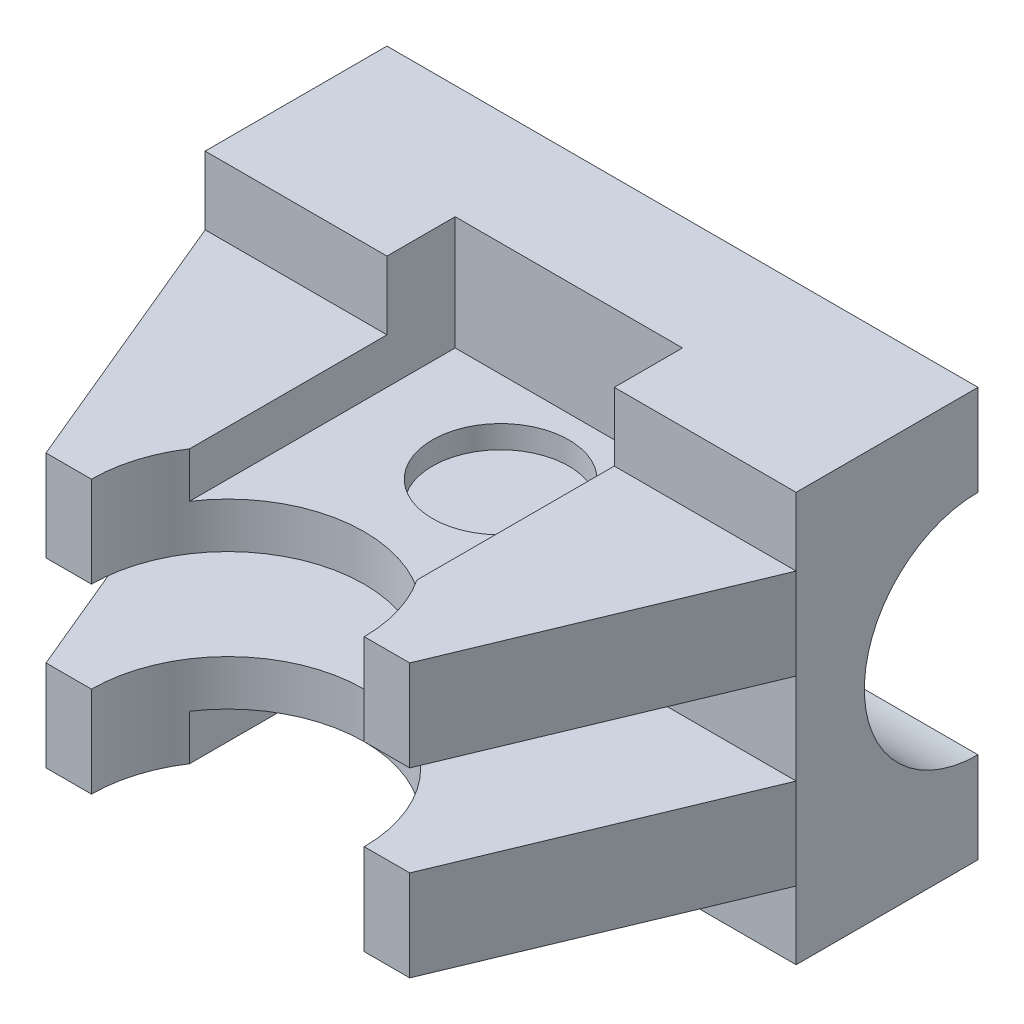
ISO-10303-21;
HEADER;
FILE_DESCRIPTION(('STEP AP214'),'2;1');
FILE_NAME('part.step','',(''),(''),'','','');
FILE_SCHEMA(('AUTOMOTIVE_DESIGN { 1 0 10303 214 1 1 1 1 }'));
ENDSEC;
DATA;
#1=APPLICATION_CONTEXT('core data for automotive mechanical design processes');
#2=APPLICATION_PROTOCOL_DEFINITION('international standard','automotive_design',2000,#1);
#3=PRODUCT_CONTEXT('',#1,'mechanical');
#4=PRODUCT('Part','Part','',(#3));
#5=PRODUCT_RELATED_PRODUCT_CATEGORY('part','',(#4));
#6=PRODUCT_DEFINITION_FORMATION('','',#4);
#7=PRODUCT_DEFINITION_CONTEXT('part definition',#1,'design');
#8=PRODUCT_DEFINITION('design','',#6,#7);
#9=PRODUCT_DEFINITION_SHAPE('','',#8);
#10=(LENGTH_UNIT() NAMED_UNIT(*) SI_UNIT(.MILLI.,.METRE.));
#11=(NAMED_UNIT(*) PLANE_ANGLE_UNIT() SI_UNIT($,.RADIAN.));
#12=(NAMED_UNIT(*) SI_UNIT($,.STERADIAN.) SOLID_ANGLE_UNIT());
#13=UNCERTAINTY_MEASURE_WITH_UNIT(LENGTH_MEASURE(1.E-05),#10,'distance_accuracy_value','');
#14=(GEOMETRIC_REPRESENTATION_CONTEXT(3) GLOBAL_UNCERTAINTY_ASSIGNED_CONTEXT((#13)) GLOBAL_UNIT_ASSIGNED_CONTEXT((#10,
#11,#12)) REPRESENTATION_CONTEXT('',''));
#15=CARTESIAN_POINT('',(0.,0.,0.));
#16=DIRECTION('',(0.,0.,1.));
#17=DIRECTION('',(1.,0.,0.));
#18=AXIS2_PLACEMENT_3D('',#15,#16,#17);
#19=CARTESIAN_POINT('',(0.,0.,0.));
#20=DIRECTION('',(0.,0.,1.));
#21=DIRECTION('',(1.,0.,0.));
#22=AXIS2_PLACEMENT_3D('',#19,#20,#21);
#23=PLANE('',#22);
#24=DIRECTION('',(0.,-1.,0.));
#25=VECTOR('',#24,1.);
#26=CARTESIAN_POINT('',(0.,90.,0.));
#27=LINE('',#26,#25);
#28=CARTESIAN_POINT('',(0.,20.,0.));
#29=VERTEX_POINT('',#28);
#30=CARTESIAN_POINT('',(0.,0.,0.));
#31=VERTEX_POINT('',#30);
#32=EDGE_CURVE('E250',#29,#31,#27,.T.);
#33=ORIENTED_EDGE('',*,*,#32,.F.);
#34=DIRECTION('',(1.,0.,0.));
#35=VECTOR('',#34,1.);
#36=CARTESIAN_POINT('',(0.,20.,0.));
#37=LINE('',#36,#35);
#38=CARTESIAN_POINT('',(130.,20.,0.));
#39=VERTEX_POINT('',#38);
#40=EDGE_CURVE('E234',#29,#39,#37,.T.);
#41=ORIENTED_EDGE('',*,*,#40,.T.);
#42=DIRECTION('',(0.,1.,0.));
#43=VECTOR('',#42,1.);
#44=CARTESIAN_POINT('',(130.,0.,0.));
#45=LINE('',#44,#43);
#46=CARTESIAN_POINT('',(130.,0.,0.));
#47=VERTEX_POINT('',#46);
#48=EDGE_CURVE('E262',#47,#39,#45,.T.);
#49=ORIENTED_EDGE('',*,*,#48,.F.);
#50=DIRECTION('',(1.,0.,0.));
#51=VECTOR('',#50,1.);
#52=CARTESIAN_POINT('',(0.,0.,0.));
#53=LINE('',#52,#51);
#54=EDGE_CURVE('E254',#31,#47,#53,.T.);
#55=ORIENTED_EDGE('',*,*,#54,.F.);
#56=EDGE_LOOP('',(#33,#41,#49,#55));
#57=FACE_BOUND('',#56,.T.);
#58=ADVANCED_FACE('F39',(#57),#23,.F.);
#59=CARTESIAN_POINT('',(65.,75.,100.));
#60=DIRECTION('',(0.,0.,1.));
#61=DIRECTION('',(1.,0.,0.));
#62=AXIS2_PLACEMENT_3D('',#59,#60,#61);
#63=PLANE('',#62);
#64=DIRECTION('',(1.,0.,0.));
#65=VECTOR('',#64,1.);
#66=CARTESIAN_POINT('',(130.,35.,100.));
#67=LINE('',#66,#65);
#68=CARTESIAN_POINT('',(25.,35.,100.));
#69=VERTEX_POINT('',#68);
#70=CARTESIAN_POINT('',(35.,35.,100.));
#71=VERTEX_POINT('',#70);
#72=EDGE_CURVE('E473',#69,#71,#67,.T.);
#73=ORIENTED_EDGE('',*,*,#72,.F.);
#74=DIRECTION('',(0.,-1.,0.));
#75=VECTOR('',#74,1.);
#76=CARTESIAN_POINT('',(25.,75.,100.));
#77=LINE('',#76,#75);
#78=CARTESIAN_POINT('',(25.,15.,100.));
#79=VERTEX_POINT('',#78);
#80=EDGE_CURVE('E347',#69,#79,#77,.T.);
#81=ORIENTED_EDGE('',*,*,#80,.T.);
#82=DIRECTION('',(-1.,0.,0.));
#83=VECTOR('',#82,1.);
#84=CARTESIAN_POINT('',(25.,15.,100.));
#85=LINE('',#84,#83);
#86=CARTESIAN_POINT('',(35.,15.,100.));
#87=VERTEX_POINT('',#86);
#88=EDGE_CURVE('E335',#87,#79,#85,.T.);
#89=ORIENTED_EDGE('',*,*,#88,.F.);
#90=DIRECTION('',(0.,-1.,0.));
#91=VECTOR('',#90,1.);
#92=CARTESIAN_POINT('',(35.,85.,100.));
#93=LINE('',#92,#91);
#94=EDGE_CURVE('E300',#71,#87,#93,.T.);
#95=ORIENTED_EDGE('',*,*,#94,.F.);
#96=EDGE_LOOP('',(#73,#81,#89,#95));
#97=FACE_BOUND('',#96,.T.);
#98=ADVANCED_FACE('F609',(#97),#63,.T.);
#99=CARTESIAN_POINT('',(95.,35.,100.));
#100=VERTEX_POINT('',#99);
#101=CARTESIAN_POINT('',(105.,35.,100.));
#102=VERTEX_POINT('',#101);
#103=EDGE_CURVE('E472',#100,#102,#67,.T.);
#104=ORIENTED_EDGE('',*,*,#103,.F.);
#105=DIRECTION('',(0.,-1.,0.));
#106=VECTOR('',#105,1.);
#107=CARTESIAN_POINT('',(95.,85.,100.));
#108=LINE('',#107,#106);
#109=CARTESIAN_POINT('',(95.,15.,100.));
#110=VERTEX_POINT('',#109);
#111=EDGE_CURVE('E296',#100,#110,#108,.T.);
#112=ORIENTED_EDGE('',*,*,#111,.T.);
#113=CARTESIAN_POINT('',(105.,15.,100.));
#114=VERTEX_POINT('',#113);
#115=EDGE_CURVE('E334',#114,#110,#85,.T.);
#116=ORIENTED_EDGE('',*,*,#115,.F.);
#117=DIRECTION('',(0.,-1.,0.));
#118=VECTOR('',#117,1.);
#119=CARTESIAN_POINT('',(105.,75.,100.));
#120=LINE('',#119,#118);
#121=EDGE_CURVE('E351',#102,#114,#120,.T.);
#122=ORIENTED_EDGE('',*,*,#121,.F.);
#123=EDGE_LOOP('',(#104,#112,#116,#122));
#124=FACE_BOUND('',#123,.T.);
#125=ADVANCED_FACE('F614',(#124),#63,.T.);
#126=CARTESIAN_POINT('',(105.,75.,100.));
#127=DIRECTION('',(0.923076923076923,0.,0.384615384615385));
#128=DIRECTION('',(0.384615384615385,0.,-0.923076923076923));
#129=AXIS2_PLACEMENT_3D('',#126,#127,#128);
#130=PLANE('',#129);
#131=DIRECTION('',(0.384615384615385,0.,-0.923076923076923));
#132=VECTOR('',#131,1.);
#133=CARTESIAN_POINT('',(105.,35.,100.));
#134=LINE('',#133,#132);
#135=CARTESIAN_POINT('',(130.,35.,40.));
#136=VERTEX_POINT('',#135);
#137=EDGE_CURVE('E478',#102,#136,#134,.T.);
#138=ORIENTED_EDGE('',*,*,#137,.F.);
#139=ORIENTED_EDGE('',*,*,#121,.T.);
#140=DIRECTION('',(-0.384615384615385,0.,0.923076923076923));
#141=VECTOR('',#140,1.);
#142=CARTESIAN_POINT('',(105.,15.,100.));
#143=LINE('',#142,#141);
#144=CARTESIAN_POINT('',(130.,15.,40.));
#145=VERTEX_POINT('',#144);
#146=EDGE_CURVE('E328',#145,#114,#143,.T.);
#147=ORIENTED_EDGE('',*,*,#146,.F.);
#148=DIRECTION('',(0.,-1.,0.));
#149=VECTOR('',#148,1.);
#150=CARTESIAN_POINT('',(130.,75.,40.));
#151=LINE('',#150,#149);
#152=EDGE_CURVE('E356',#136,#145,#151,.T.);
#153=ORIENTED_EDGE('',*,*,#152,.F.);
#154=EDGE_LOOP('',(#138,#139,#147,#153));
#155=FACE_BOUND('',#154,.T.);
#156=ADVANCED_FACE('F598',(#155),#130,.T.);
#157=CARTESIAN_POINT('',(25.,75.,100.));
#158=DIRECTION('',(-0.923076923076923,0.,0.384615384615385));
#159=DIRECTION('',(0.384615384615385,0.,0.923076923076923));
#160=AXIS2_PLACEMENT_3D('',#157,#158,#159);
#161=PLANE('',#160);
#162=DIRECTION('',(0.384615384615385,0.,0.923076923076923));
#163=VECTOR('',#162,1.);
#164=CARTESIAN_POINT('',(25.,35.,100.));
#165=LINE('',#164,#163);
#166=CARTESIAN_POINT('',(0.,35.,40.));
#167=VERTEX_POINT('',#166);
#168=EDGE_CURVE('E476',#167,#69,#165,.T.);
#169=ORIENTED_EDGE('',*,*,#168,.F.);
#170=DIRECTION('',(0.,-1.,0.));
#171=VECTOR('',#170,1.);
#172=CARTESIAN_POINT('',(0.,90.,40.));
#173=LINE('',#172,#171);
#174=CARTESIAN_POINT('',(0.,15.,40.));
#175=VERTEX_POINT('',#174);
#176=EDGE_CURVE('E415',#167,#175,#173,.T.);
#177=ORIENTED_EDGE('',*,*,#176,.T.);
#178=DIRECTION('',(-0.384615384615385,0.,-0.923076923076923));
#179=VECTOR('',#178,1.);
#180=CARTESIAN_POINT('',(0.,15.,40.));
#181=LINE('',#180,#179);
#182=EDGE_CURVE('E337',#79,#175,#181,.T.);
#183=ORIENTED_EDGE('',*,*,#182,.F.);
#184=ORIENTED_EDGE('',*,*,#80,.F.);
#185=EDGE_LOOP('',(#169,#177,#183,#184));
#186=FACE_BOUND('',#185,.T.);
#187=ADVANCED_FACE('F566',(#186),#161,.T.);
#188=CARTESIAN_POINT('',(65.,85.,100.));
#189=DIRECTION('',(0.,-1.,0.));
#190=DIRECTION('',(0.,0.,-1.));
#191=AXIS2_PLACEMENT_3D('',#188,#189,#190);
#192=CYLINDRICAL_SURFACE('',#191,30.);
#193=ORIENTED_EDGE('',*,*,#111,.F.);
#194=CARTESIAN_POINT('',(65.,35.,100.));
#195=DIRECTION('',(0.,-1.,0.));
#196=DIRECTION('',(0.,0.,-1.));
#197=AXIS2_PLACEMENT_3D('',#194,#195,#196);
#198=CIRCLE('',#197,30.);
#199=EDGE_CURVE('E11',#100,#71,#198,.F.);
#200=ORIENTED_EDGE('',*,*,#199,.T.);
#201=ORIENTED_EDGE('',*,*,#94,.T.);
#202=CARTESIAN_POINT('',(65.,15.,100.));
#203=DIRECTION('',(0.,1.,0.));
#204=DIRECTION('',(0.,0.,1.));
#205=AXIS2_PLACEMENT_3D('',#202,#203,#204);
#206=CIRCLE('',#205,30.);
#207=CARTESIAN_POINT('',(40.,15.,83.416876048223));
#208=VERTEX_POINT('',#207);
#209=EDGE_CURVE('E481',#208,#87,#206,.T.);
#210=ORIENTED_EDGE('',*,*,#209,.F.);
#211=DIRECTION('',(0.,1.,0.));
#212=VECTOR('',#211,1.);
#213=CARTESIAN_POINT('',(40.,-35.,83.416876048223));
#214=LINE('',#213,#212);
#215=CARTESIAN_POINT('',(40.,25.,83.416876048223));
#216=VERTEX_POINT('',#215);
#217=EDGE_CURVE('E485',#208,#216,#214,.T.);
#218=ORIENTED_EDGE('',*,*,#217,.T.);
#219=CARTESIAN_POINT('',(65.,25.,100.));
#220=DIRECTION('',(0.,-1.,0.));
#221=DIRECTION('',(0.,0.,-1.));
#222=AXIS2_PLACEMENT_3D('',#219,#220,#221);
#223=CIRCLE('',#222,30.);
#224=CARTESIAN_POINT('',(90.,25.,83.416876048223));
#225=VERTEX_POINT('',#224);
#226=EDGE_CURVE('E301',#216,#225,#223,.T.);
#227=ORIENTED_EDGE('',*,*,#226,.T.);
#228=DIRECTION('',(0.,1.,0.));
#229=VECTOR('',#228,1.);
#230=CARTESIAN_POINT('',(90.,-35.,83.416876048223));
#231=LINE('',#230,#229);
#232=CARTESIAN_POINT('',(90.,15.,83.416876048223));
#233=VERTEX_POINT('',#232);
#234=EDGE_CURVE('E482',#233,#225,#231,.T.);
#235=ORIENTED_EDGE('',*,*,#234,.F.);
#236=CARTESIAN_POINT('',(65.,15.,100.));
#237=DIRECTION('',(0.,1.,0.));
#238=DIRECTION('',(0.,0.,1.));
#239=AXIS2_PLACEMENT_3D('',#236,#237,#238);
#240=CIRCLE('',#239,30.);
#241=EDGE_CURVE('E486',#110,#233,#240,.T.);
#242=ORIENTED_EDGE('',*,*,#241,.F.);
#243=EDGE_LOOP('',(#193,#200,#201,#210,#218,#227,#235,#242));
#244=FACE_BOUND('',#243,.T.);
#245=ADVANCED_FACE('F494',(#244),#192,.F.);
#246=DIRECTION('',(-1.,0.,0.));
#247=VECTOR('',#246,1.);
#248=CARTESIAN_POINT('',(0.,55.,100.));
#249=LINE('',#248,#247);
#250=CARTESIAN_POINT('',(35.,55.,100.));
#251=VERTEX_POINT('',#250);
#252=CARTESIAN_POINT('',(25.,55.,100.));
#253=VERTEX_POINT('',#252);
#254=EDGE_CURVE('E468',#251,#253,#249,.T.);
#255=ORIENTED_EDGE('',*,*,#254,.F.);
#256=CARTESIAN_POINT('',(35.,75.,100.));
#257=VERTEX_POINT('',#256);
#258=EDGE_CURVE('E286',#257,#251,#93,.T.);
#259=ORIENTED_EDGE('',*,*,#258,.F.);
#260=DIRECTION('',(-1.,0.,0.));
#261=VECTOR('',#260,1.);
#262=CARTESIAN_POINT('',(65.,75.,100.));
#263=LINE('',#262,#261);
#264=CARTESIAN_POINT('',(25.,75.,100.));
#265=VERTEX_POINT('',#264);
#266=EDGE_CURVE('E339',#257,#265,#263,.T.);
#267=ORIENTED_EDGE('',*,*,#266,.T.);
#268=EDGE_CURVE('E360',#265,#253,#77,.T.);
#269=ORIENTED_EDGE('',*,*,#268,.T.);
#270=EDGE_LOOP('',(#255,#259,#267,#269));
#271=FACE_BOUND('',#270,.T.);
#272=ADVANCED_FACE('F539',(#271),#63,.T.);
#273=CARTESIAN_POINT('',(105.,55.,100.));
#274=VERTEX_POINT('',#273);
#275=CARTESIAN_POINT('',(95.,55.,100.));
#276=VERTEX_POINT('',#275);
#277=EDGE_CURVE('E65',#274,#276,#249,.T.);
#278=ORIENTED_EDGE('',*,*,#277,.F.);
#279=CARTESIAN_POINT('',(105.,75.,100.));
#280=VERTEX_POINT('',#279);
#281=EDGE_CURVE('E352',#280,#274,#120,.T.);
#282=ORIENTED_EDGE('',*,*,#281,.F.);
#283=CARTESIAN_POINT('',(95.,75.,100.));
#284=VERTEX_POINT('',#283);
#285=EDGE_CURVE('E298',#280,#284,#263,.T.);
#286=ORIENTED_EDGE('',*,*,#285,.T.);
#287=EDGE_CURVE('E287',#284,#276,#108,.T.);
#288=ORIENTED_EDGE('',*,*,#287,.T.);
#289=EDGE_LOOP('',(#278,#282,#286,#288));
#290=FACE_BOUND('',#289,.T.);
#291=ADVANCED_FACE('F291',(#290),#63,.T.);
#292=CARTESIAN_POINT('',(0.,75.,0.));
#293=DIRECTION('',(0.,-1.,0.));
#294=DIRECTION('',(0.,0.,-1.));
#295=AXIS2_PLACEMENT_3D('',#292,#293,#294);
#296=PLANE('',#295);
#297=ORIENTED_EDGE('',*,*,#266,.F.);
#298=CARTESIAN_POINT('',(65.,75.,100.));
#299=DIRECTION('',(0.,-1.,0.));
#300=DIRECTION('',(0.,0.,-1.));
#301=AXIS2_PLACEMENT_3D('',#298,#299,#300);
#302=CIRCLE('',#301,30.);
#303=CARTESIAN_POINT('',(40.,75.,83.416876048223));
#304=VERTEX_POINT('',#303);
#305=EDGE_CURVE('E315',#257,#304,#302,.T.);
#306=ORIENTED_EDGE('',*,*,#305,.T.);
#307=DIRECTION('',(0.,0.,-1.));
#308=VECTOR('',#307,1.);
#309=CARTESIAN_POINT('',(40.,75.,0.));
#310=LINE('',#309,#308);
#311=CARTESIAN_POINT('',(40.,75.,40.));
#312=VERTEX_POINT('',#311);
#313=EDGE_CURVE('E314',#304,#312,#310,.T.);
#314=ORIENTED_EDGE('',*,*,#313,.T.);
#315=DIRECTION('',(1.,0.,0.));
#316=VECTOR('',#315,1.);
#317=CARTESIAN_POINT('',(130.,75.,40.));
#318=LINE('',#317,#316);
#319=CARTESIAN_POINT('',(0.,75.,40.));
#320=VERTEX_POINT('',#319);
#321=EDGE_CURVE('E343',#320,#312,#318,.T.);
#322=ORIENTED_EDGE('',*,*,#321,.F.);
#323=DIRECTION('',(-0.384615384615385,0.,-0.923076923076923));
#324=VECTOR('',#323,1.);
#325=CARTESIAN_POINT('',(25.,75.,100.));
#326=LINE('',#325,#324);
#327=EDGE_CURVE('E341',#265,#320,#326,.T.);
#328=ORIENTED_EDGE('',*,*,#327,.F.);
#329=EDGE_LOOP('',(#297,#306,#314,#322,#328));
#330=FACE_BOUND('',#329,.T.);
#331=ADVANCED_FACE('F540',(#330),#296,.F.);
#332=DIRECTION('',(0.,0.,1.));
#333=VECTOR('',#332,1.);
#334=CARTESIAN_POINT('',(90.,75.,0.));
#335=LINE('',#334,#333);
#336=CARTESIAN_POINT('',(90.,75.,40.));
#337=VERTEX_POINT('',#336);
#338=CARTESIAN_POINT('',(90.,75.,83.416876048223));
#339=VERTEX_POINT('',#338);
#340=EDGE_CURVE('E320',#337,#339,#335,.T.);
#341=ORIENTED_EDGE('',*,*,#340,.T.);
#342=CARTESIAN_POINT('',(65.,75.,100.));
#343=DIRECTION('',(0.,-1.,0.));
#344=DIRECTION('',(0.,0.,-1.));
#345=AXIS2_PLACEMENT_3D('',#342,#343,#344);
#346=CIRCLE('',#345,30.);
#347=EDGE_CURVE('E309',#339,#284,#346,.T.);
#348=ORIENTED_EDGE('',*,*,#347,.T.);
#349=ORIENTED_EDGE('',*,*,#285,.F.);
#350=DIRECTION('',(-0.384615384615385,0.,0.923076923076923));
#351=VECTOR('',#350,1.);
#352=CARTESIAN_POINT('',(105.,75.,100.));
#353=LINE('',#352,#351);
#354=CARTESIAN_POINT('',(130.,75.,40.));
#355=VERTEX_POINT('',#354);
#356=EDGE_CURVE('E346',#355,#280,#353,.T.);
#357=ORIENTED_EDGE('',*,*,#356,.F.);
#358=EDGE_CURVE('E279',#337,#355,#318,.T.);
#359=ORIENTED_EDGE('',*,*,#358,.F.);
#360=EDGE_LOOP('',(#341,#348,#349,#357,#359));
#361=FACE_BOUND('',#360,.T.);
#362=ADVANCED_FACE('F446',(#361),#296,.F.);
#363=CARTESIAN_POINT('',(0.,15.,0.));
#364=DIRECTION('',(0.,1.,0.));
#365=DIRECTION('',(0.,0.,1.));
#366=AXIS2_PLACEMENT_3D('',#363,#364,#365);
#367=PLANE('',#366);
#368=ORIENTED_EDGE('',*,*,#115,.T.);
#369=ORIENTED_EDGE('',*,*,#241,.T.);
#370=DIRECTION('',(0.,0.,1.));
#371=VECTOR('',#370,1.);
#372=CARTESIAN_POINT('',(90.,15.,0.));
#373=LINE('',#372,#371);
#374=CARTESIAN_POINT('',(90.,15.,40.));
#375=VERTEX_POINT('',#374);
#376=EDGE_CURVE('E325',#375,#233,#373,.T.);
#377=ORIENTED_EDGE('',*,*,#376,.F.);
#378=DIRECTION('',(1.,0.,0.));
#379=VECTOR('',#378,1.);
#380=CARTESIAN_POINT('',(40.,15.,40.));
#381=LINE('',#380,#379);
#382=EDGE_CURVE('E324',#375,#145,#381,.T.);
#383=ORIENTED_EDGE('',*,*,#382,.T.);
#384=ORIENTED_EDGE('',*,*,#146,.T.);
#385=EDGE_LOOP('',(#368,#369,#377,#383,#384));
#386=FACE_BOUND('',#385,.T.);
#387=ADVANCED_FACE('F506',(#386),#367,.F.);
#388=CARTESIAN_POINT('',(0.,0.,40.));
#389=DIRECTION('',(0.,0.,1.));
#390=DIRECTION('',(1.,0.,0.));
#391=AXIS2_PLACEMENT_3D('',#388,#389,#390);
#392=PLANE('',#391);
#393=DIRECTION('',(0.,-1.,0.));
#394=VECTOR('',#393,1.);
#395=CARTESIAN_POINT('',(40.,25.,40.));
#396=LINE('',#395,#394);
#397=CARTESIAN_POINT('',(40.,15.,40.));
#398=VERTEX_POINT('',#397);
#399=CARTESIAN_POINT('',(40.,0.,40.));
#400=VERTEX_POINT('',#399);
#401=EDGE_CURVE('E397',#398,#400,#396,.T.);
#402=ORIENTED_EDGE('',*,*,#401,.F.);
#403=EDGE_CURVE('E329',#175,#398,#381,.T.);
#404=ORIENTED_EDGE('',*,*,#403,.F.);
#405=CARTESIAN_POINT('',(0.,0.,40.));
#406=VERTEX_POINT('',#405);
#407=EDGE_CURVE('E266',#175,#406,#173,.T.);
#408=ORIENTED_EDGE('',*,*,#407,.T.);
#409=DIRECTION('',(1.,0.,0.));
#410=VECTOR('',#409,1.);
#411=CARTESIAN_POINT('',(0.,0.,40.));
#412=LINE('',#411,#410);
#413=EDGE_CURVE('E413',#406,#400,#412,.T.);
#414=ORIENTED_EDGE('',*,*,#413,.T.);
#415=EDGE_LOOP('',(#402,#404,#408,#414));
#416=FACE_BOUND('',#415,.T.);
#417=ADVANCED_FACE('F553',(#416),#392,.T.);
#418=DIRECTION('',(0.,1.,0.));
#419=VECTOR('',#418,1.);
#420=CARTESIAN_POINT('',(130.,0.,40.));
#421=LINE('',#420,#419);
#422=CARTESIAN_POINT('',(130.,0.,40.));
#423=VERTEX_POINT('',#422);
#424=EDGE_CURVE('E420',#423,#145,#421,.T.);
#425=ORIENTED_EDGE('',*,*,#424,.T.);
#426=ORIENTED_EDGE('',*,*,#382,.F.);
#427=DIRECTION('',(0.,-1.,0.));
#428=VECTOR('',#427,1.);
#429=CARTESIAN_POINT('',(90.,25.,40.));
#430=LINE('',#429,#428);
#431=CARTESIAN_POINT('',(90.,0.,40.));
#432=VERTEX_POINT('',#431);
#433=EDGE_CURVE('E253',#375,#432,#430,.T.);
#434=ORIENTED_EDGE('',*,*,#433,.T.);
#435=EDGE_CURVE('E414',#432,#423,#412,.T.);
#436=ORIENTED_EDGE('',*,*,#435,.T.);
#437=EDGE_LOOP('',(#425,#426,#434,#436));
#438=FACE_BOUND('',#437,.T.);
#439=ADVANCED_FACE('F507',(#438),#392,.T.);
#440=CARTESIAN_POINT('',(0.,25.,0.));
#441=DIRECTION('',(0.,-1.,0.));
#442=DIRECTION('',(0.,0.,-1.));
#443=AXIS2_PLACEMENT_3D('',#440,#441,#442);
#444=PLANE('',#443);
#445=CARTESIAN_POINT('',(60.,25.,45.));
#446=DIRECTION('',(0.,-1.,0.));
#447=DIRECTION('',(0.,0.,-1.));
#448=AXIS2_PLACEMENT_3D('',#445,#446,#447);
#449=CIRCLE('',#448,15.);
#450=CARTESIAN_POINT('',(60.,25.,30.));
#451=VERTEX_POINT('',#450);
#452=EDGE_CURVE('E571',#451,#451,#449,.T.);
#453=ORIENTED_EDGE('',*,*,#452,.F.);
#454=EDGE_LOOP('',(#453));
#455=FACE_BOUND('',#454,.T.);
#456=ORIENTED_EDGE('',*,*,#226,.F.);
#457=DIRECTION('',(0.,0.,-1.));
#458=VECTOR('',#457,1.);
#459=CARTESIAN_POINT('',(40.,25.,40.));
#460=LINE('',#459,#458);
#461=CARTESIAN_POINT('',(40.,25.,25.));
#462=VERTEX_POINT('',#461);
#463=EDGE_CURVE('E390',#216,#462,#460,.T.);
#464=ORIENTED_EDGE('',*,*,#463,.T.);
#465=DIRECTION('',(1.,0.,0.));
#466=VECTOR('',#465,1.);
#467=CARTESIAN_POINT('',(40.,25.,25.));
#468=LINE('',#467,#466);
#469=CARTESIAN_POINT('',(90.,25.,25.));
#470=VERTEX_POINT('',#469);
#471=EDGE_CURVE('E388',#462,#470,#468,.T.);
#472=ORIENTED_EDGE('',*,*,#471,.T.);
#473=DIRECTION('',(0.,0.,1.));
#474=VECTOR('',#473,1.);
#475=CARTESIAN_POINT('',(90.,25.,25.));
#476=LINE('',#475,#474);
#477=EDGE_CURVE('E395',#470,#225,#476,.T.);
#478=ORIENTED_EDGE('',*,*,#477,.T.);
#479=EDGE_LOOP('',(#456,#464,#472,#478));
#480=FACE_BOUND('',#479,.T.);
#481=ADVANCED_FACE('F499',(#455,#480),#444,.T.);
#482=CARTESIAN_POINT('',(0.,90.,40.));
#483=VERTEX_POINT('',#482);
#484=EDGE_CURVE('E407',#483,#320,#173,.T.);
#485=ORIENTED_EDGE('',*,*,#484,.T.);
#486=ORIENTED_EDGE('',*,*,#321,.T.);
#487=DIRECTION('',(0.,1.,0.));
#488=VECTOR('',#487,1.);
#489=CARTESIAN_POINT('',(40.,65.,40.));
#490=LINE('',#489,#488);
#491=CARTESIAN_POINT('',(40.,90.,40.));
#492=VERTEX_POINT('',#491);
#493=EDGE_CURVE('E378',#312,#492,#490,.T.);
#494=ORIENTED_EDGE('',*,*,#493,.T.);
#495=DIRECTION('',(-1.,0.,0.));
#496=VECTOR('',#495,1.);
#497=CARTESIAN_POINT('',(130.,90.,40.));
#498=LINE('',#497,#496);
#499=EDGE_CURVE('E416',#492,#483,#498,.T.);
#500=ORIENTED_EDGE('',*,*,#499,.T.);
#501=EDGE_LOOP('',(#485,#486,#494,#500));
#502=FACE_BOUND('',#501,.T.);
#503=ADVANCED_FACE('F523',(#502),#392,.T.);
#504=DIRECTION('',(0.,1.,0.));
#505=VECTOR('',#504,1.);
#506=CARTESIAN_POINT('',(90.,65.,40.));
#507=LINE('',#506,#505);
#508=CARTESIAN_POINT('',(90.,90.,40.));
#509=VERTEX_POINT('',#508);
#510=EDGE_CURVE('E371',#337,#509,#507,.T.);
#511=ORIENTED_EDGE('',*,*,#510,.F.);
#512=ORIENTED_EDGE('',*,*,#358,.T.);
#513=CARTESIAN_POINT('',(130.,90.,40.));
#514=VERTEX_POINT('',#513);
#515=EDGE_CURVE('E417',#355,#514,#421,.T.);
#516=ORIENTED_EDGE('',*,*,#515,.T.);
#517=EDGE_CURVE('E264',#514,#509,#498,.T.);
#518=ORIENTED_EDGE('',*,*,#517,.T.);
#519=EDGE_LOOP('',(#511,#512,#516,#518));
#520=FACE_BOUND('',#519,.T.);
#521=ADVANCED_FACE('F427',(#520),#392,.T.);
#522=CARTESIAN_POINT('',(0.,90.,40.));
#523=DIRECTION('',(1.,0.,0.));
#524=DIRECTION('',(0.,0.,-1.));
#525=AXIS2_PLACEMENT_3D('',#522,#523,#524);
#526=PLANE('',#525);
#527=CARTESIAN_POINT('',(0.,90.,0.));
#528=VERTEX_POINT('',#527);
#529=CARTESIAN_POINT('',(0.,70.,0.));
#530=VERTEX_POINT('',#529);
#531=EDGE_CURVE('E252',#528,#530,#27,.T.);
#532=ORIENTED_EDGE('',*,*,#531,.T.);
#533=CARTESIAN_POINT('',(0.,45.,0.));
#534=DIRECTION('',(1.,0.,0.));
#535=DIRECTION('',(0.,0.,-1.));
#536=AXIS2_PLACEMENT_3D('',#533,#534,#535);
#537=CIRCLE('',#536,25.);
#538=EDGE_CURVE('E53',#530,#29,#537,.T.);
#539=ORIENTED_EDGE('',*,*,#538,.T.);
#540=ORIENTED_EDGE('',*,*,#32,.T.);
#541=DIRECTION('',(0.,0.,-1.));
#542=VECTOR('',#541,1.);
#543=CARTESIAN_POINT('',(0.,0.,40.));
#544=LINE('',#543,#542);
#545=EDGE_CURVE('E277',#406,#31,#544,.T.);
#546=ORIENTED_EDGE('',*,*,#545,.F.);
#547=ORIENTED_EDGE('',*,*,#407,.F.);
#548=ORIENTED_EDGE('',*,*,#176,.F.);
#549=DIRECTION('',(0.,-1.,0.));
#550=VECTOR('',#549,1.);
#551=CARTESIAN_POINT('',(0.,35.,40.));
#552=LINE('',#551,#550);
#553=CARTESIAN_POINT('',(0.,55.,40.));
#554=VERTEX_POINT('',#553);
#555=EDGE_CURVE('E467',#554,#167,#552,.T.);
#556=ORIENTED_EDGE('',*,*,#555,.F.);
#557=EDGE_CURVE('E411',#320,#554,#173,.T.);
#558=ORIENTED_EDGE('',*,*,#557,.F.);
#559=ORIENTED_EDGE('',*,*,#484,.F.);
#560=DIRECTION('',(0.,0.,-1.));
#561=VECTOR('',#560,1.);
#562=CARTESIAN_POINT('',(0.,90.,40.));
#563=LINE('',#562,#561);
#564=EDGE_CURVE('E268',#483,#528,#563,.T.);
#565=ORIENTED_EDGE('',*,*,#564,.T.);
#566=EDGE_LOOP('',(#532,#539,#540,#546,#547,#548,#556,#558,#559,#565));
#567=FACE_BOUND('',#566,.T.);
#568=ADVANCED_FACE('F41',(#567),#526,.F.);
#569=CARTESIAN_POINT('',(0.,0.,40.));
#570=DIRECTION('',(0.,1.,0.));
#571=DIRECTION('',(0.,0.,1.));
#572=AXIS2_PLACEMENT_3D('',#569,#570,#571);
#573=PLANE('',#572);
#574=ORIENTED_EDGE('',*,*,#435,.F.);
#575=DIRECTION('',(0.,0.,1.));
#576=VECTOR('',#575,1.);
#577=CARTESIAN_POINT('',(90.,0.,25.));
#578=LINE('',#577,#576);
#579=CARTESIAN_POINT('',(90.,0.,25.));
#580=VERTEX_POINT('',#579);
#581=EDGE_CURVE('E389',#580,#432,#578,.T.);
#582=ORIENTED_EDGE('',*,*,#581,.F.);
#583=DIRECTION('',(1.,0.,0.));
#584=VECTOR('',#583,1.);
#585=CARTESIAN_POINT('',(40.,0.,25.));
#586=LINE('',#585,#584);
#587=CARTESIAN_POINT('',(40.,0.,25.));
#588=VERTEX_POINT('',#587);
#589=EDGE_CURVE('E396',#588,#580,#586,.T.);
#590=ORIENTED_EDGE('',*,*,#589,.F.);
#591=DIRECTION('',(0.,0.,-1.));
#592=VECTOR('',#591,1.);
#593=CARTESIAN_POINT('',(40.,0.,40.));
#594=LINE('',#593,#592);
#595=EDGE_CURVE('E382',#400,#588,#594,.T.);
#596=ORIENTED_EDGE('',*,*,#595,.F.);
#597=ORIENTED_EDGE('',*,*,#413,.F.);
#598=ORIENTED_EDGE('',*,*,#545,.T.);
#599=ORIENTED_EDGE('',*,*,#54,.T.);
#600=DIRECTION('',(0.,0.,-1.));
#601=VECTOR('',#600,1.);
#602=CARTESIAN_POINT('',(130.,0.,40.));
#603=LINE('',#602,#601);
#604=EDGE_CURVE('E273',#423,#47,#603,.T.);
#605=ORIENTED_EDGE('',*,*,#604,.F.);
#606=EDGE_LOOP('',(#574,#582,#590,#596,#597,#598,#599,#605));
#607=FACE_BOUND('',#606,.T.);
#608=ADVANCED_FACE('F511',(#607),#573,.F.);
#609=CARTESIAN_POINT('',(130.,0.,40.));
#610=DIRECTION('',(-1.,0.,0.));
#611=DIRECTION('',(0.,0.,1.));
#612=AXIS2_PLACEMENT_3D('',#609,#610,#611);
#613=PLANE('',#612);
#614=ORIENTED_EDGE('',*,*,#48,.T.);
#615=CARTESIAN_POINT('',(130.,45.,0.));
#616=DIRECTION('',(1.,0.,0.));
#617=DIRECTION('',(0.,0.,-1.));
#618=AXIS2_PLACEMENT_3D('',#615,#616,#617);
#619=CIRCLE('',#618,25.);
#620=CARTESIAN_POINT('',(130.,70.,0.));
#621=VERTEX_POINT('',#620);
#622=EDGE_CURVE('E240',#621,#39,#619,.T.);
#623=ORIENTED_EDGE('',*,*,#622,.F.);
#624=CARTESIAN_POINT('',(130.,90.,0.));
#625=VERTEX_POINT('',#624);
#626=EDGE_CURVE('E263',#621,#625,#45,.T.);
#627=ORIENTED_EDGE('',*,*,#626,.T.);
#628=DIRECTION('',(0.,0.,-1.));
#629=VECTOR('',#628,1.);
#630=CARTESIAN_POINT('',(130.,90.,40.));
#631=LINE('',#630,#629);
#632=EDGE_CURVE('E275',#514,#625,#631,.T.);
#633=ORIENTED_EDGE('',*,*,#632,.F.);
#634=ORIENTED_EDGE('',*,*,#515,.F.);
#635=CARTESIAN_POINT('',(130.,55.,40.));
#636=VERTEX_POINT('',#635);
#637=EDGE_CURVE('E353',#355,#636,#151,.T.);
#638=ORIENTED_EDGE('',*,*,#637,.T.);
#639=DIRECTION('',(0.,1.,0.));
#640=VECTOR('',#639,1.);
#641=CARTESIAN_POINT('',(130.,55.,40.));
#642=LINE('',#641,#640);
#643=EDGE_CURVE('E456',#136,#636,#642,.T.);
#644=ORIENTED_EDGE('',*,*,#643,.F.);
#645=ORIENTED_EDGE('',*,*,#152,.T.);
#646=ORIENTED_EDGE('',*,*,#424,.F.);
#647=ORIENTED_EDGE('',*,*,#604,.T.);
#648=EDGE_LOOP('',(#614,#623,#627,#633,#634,#638,#644,#645,#646,#647));
#649=FACE_BOUND('',#648,.T.);
#650=ADVANCED_FACE('F432',(#649),#613,.F.);
#651=CARTESIAN_POINT('',(130.,90.,40.));
#652=DIRECTION('',(0.,-1.,0.));
#653=DIRECTION('',(0.,0.,-1.));
#654=AXIS2_PLACEMENT_3D('',#651,#652,#653);
#655=PLANE('',#654);
#656=ORIENTED_EDGE('',*,*,#499,.F.);
#657=DIRECTION('',(0.,0.,1.));
#658=VECTOR('',#657,1.);
#659=CARTESIAN_POINT('',(40.,90.,25.));
#660=LINE('',#659,#658);
#661=CARTESIAN_POINT('',(40.,90.,25.));
#662=VERTEX_POINT('',#661);
#663=EDGE_CURVE('E362',#662,#492,#660,.T.);
#664=ORIENTED_EDGE('',*,*,#663,.F.);
#665=DIRECTION('',(-1.,0.,0.));
#666=VECTOR('',#665,1.);
#667=CARTESIAN_POINT('',(90.,90.,25.));
#668=LINE('',#667,#666);
#669=CARTESIAN_POINT('',(90.,90.,25.));
#670=VERTEX_POINT('',#669);
#671=EDGE_CURVE('E372',#670,#662,#668,.T.);
#672=ORIENTED_EDGE('',*,*,#671,.F.);
#673=DIRECTION('',(0.,0.,-1.));
#674=VECTOR('',#673,1.);
#675=CARTESIAN_POINT('',(90.,90.,40.));
#676=LINE('',#675,#674);
#677=EDGE_CURVE('E354',#509,#670,#676,.T.);
#678=ORIENTED_EDGE('',*,*,#677,.F.);
#679=ORIENTED_EDGE('',*,*,#517,.F.);
#680=ORIENTED_EDGE('',*,*,#632,.T.);
#681=DIRECTION('',(-1.,0.,0.));
#682=VECTOR('',#681,1.);
#683=CARTESIAN_POINT('',(130.,90.,0.));
#684=LINE('',#683,#682);
#685=EDGE_CURVE('E270',#625,#528,#684,.T.);
#686=ORIENTED_EDGE('',*,*,#685,.T.);
#687=ORIENTED_EDGE('',*,*,#564,.F.);
#688=EDGE_LOOP('',(#656,#664,#672,#678,#679,#680,#686,#687));
#689=FACE_BOUND('',#688,.T.);
#690=ADVANCED_FACE('F439',(#689),#655,.F.);
#691=ORIENTED_EDGE('',*,*,#626,.F.);
#692=DIRECTION('',(1.,0.,0.));
#693=VECTOR('',#692,1.);
#694=CARTESIAN_POINT('',(0.,70.,0.));
#695=LINE('',#694,#693);
#696=EDGE_CURVE('E245',#530,#621,#695,.T.);
#697=ORIENTED_EDGE('',*,*,#696,.F.);
#698=ORIENTED_EDGE('',*,*,#531,.F.);
#699=ORIENTED_EDGE('',*,*,#685,.F.);
#700=EDGE_LOOP('',(#691,#697,#698,#699));
#701=FACE_BOUND('',#700,.T.);
#702=ADVANCED_FACE('F520',(#701),#23,.F.);
#703=CARTESIAN_POINT('',(90.,25.,25.));
#704=DIRECTION('',(1.,0.,0.));
#705=DIRECTION('',(0.,0.,-1.));
#706=AXIS2_PLACEMENT_3D('',#703,#704,#705);
#707=PLANE('',#706);
#708=ORIENTED_EDGE('',*,*,#376,.T.);
#709=ORIENTED_EDGE('',*,*,#234,.T.);
#710=ORIENTED_EDGE('',*,*,#477,.F.);
#711=DIRECTION('',(0.,-1.,0.));
#712=VECTOR('',#711,1.);
#713=CARTESIAN_POINT('',(90.,25.,25.));
#714=LINE('',#713,#712);
#715=EDGE_CURVE('E260',#470,#580,#714,.T.);
#716=ORIENTED_EDGE('',*,*,#715,.T.);
#717=ORIENTED_EDGE('',*,*,#581,.T.);
#718=ORIENTED_EDGE('',*,*,#433,.F.);
#719=EDGE_LOOP('',(#708,#709,#710,#716,#717,#718));
#720=FACE_BOUND('',#719,.T.);
#721=ADVANCED_FACE('F503',(#720),#707,.F.);
#722=CARTESIAN_POINT('',(40.,25.,25.));
#723=DIRECTION('',(0.,0.,-1.));
#724=DIRECTION('',(-1.,0.,0.));
#725=AXIS2_PLACEMENT_3D('',#722,#723,#724);
#726=PLANE('',#725);
#727=ORIENTED_EDGE('',*,*,#589,.T.);
#728=ORIENTED_EDGE('',*,*,#715,.F.);
#729=ORIENTED_EDGE('',*,*,#471,.F.);
#730=DIRECTION('',(0.,-1.,0.));
#731=VECTOR('',#730,1.);
#732=CARTESIAN_POINT('',(40.,25.,25.));
#733=LINE('',#732,#731);
#734=EDGE_CURVE('E403',#462,#588,#733,.T.);
#735=ORIENTED_EDGE('',*,*,#734,.T.);
#736=EDGE_LOOP('',(#727,#728,#729,#735));
#737=FACE_BOUND('',#736,.T.);
#738=ADVANCED_FACE('F624',(#737),#726,.F.);
#739=CARTESIAN_POINT('',(40.,25.,40.));
#740=DIRECTION('',(-1.,0.,0.));
#741=DIRECTION('',(0.,0.,1.));
#742=AXIS2_PLACEMENT_3D('',#739,#740,#741);
#743=PLANE('',#742);
#744=ORIENTED_EDGE('',*,*,#463,.F.);
#745=ORIENTED_EDGE('',*,*,#217,.F.);
#746=DIRECTION('',(0.,0.,-1.));
#747=VECTOR('',#746,1.);
#748=CARTESIAN_POINT('',(40.,15.,0.));
#749=LINE('',#748,#747);
#750=EDGE_CURVE('E318',#208,#398,#749,.T.);
#751=ORIENTED_EDGE('',*,*,#750,.T.);
#752=ORIENTED_EDGE('',*,*,#401,.T.);
#753=ORIENTED_EDGE('',*,*,#595,.T.);
#754=ORIENTED_EDGE('',*,*,#734,.F.);
#755=EDGE_LOOP('',(#744,#745,#751,#752,#753,#754));
#756=FACE_BOUND('',#755,.T.);
#757=ADVANCED_FACE('F558',(#756),#743,.F.);
#758=CARTESIAN_POINT('',(40.,65.,25.));
#759=DIRECTION('',(-1.,0.,0.));
#760=DIRECTION('',(0.,0.,1.));
#761=AXIS2_PLACEMENT_3D('',#758,#759,#760);
#762=PLANE('',#761);
#763=ORIENTED_EDGE('',*,*,#313,.F.);
#764=DIRECTION('',(0.,-1.,0.));
#765=VECTOR('',#764,1.);
#766=CARTESIAN_POINT('',(40.,85.,83.416876048223));
#767=LINE('',#766,#765);
#768=CARTESIAN_POINT('',(40.,65.,83.416876048223));
#769=VERTEX_POINT('',#768);
#770=EDGE_CURVE('E310',#304,#769,#767,.T.);
#771=ORIENTED_EDGE('',*,*,#770,.T.);
#772=DIRECTION('',(0.,0.,1.));
#773=VECTOR('',#772,1.);
#774=CARTESIAN_POINT('',(40.,65.,25.));
#775=LINE('',#774,#773);
#776=CARTESIAN_POINT('',(40.,65.,25.));
#777=VERTEX_POINT('',#776);
#778=EDGE_CURVE('E368',#777,#769,#775,.T.);
#779=ORIENTED_EDGE('',*,*,#778,.F.);
#780=DIRECTION('',(0.,1.,0.));
#781=VECTOR('',#780,1.);
#782=CARTESIAN_POINT('',(40.,65.,25.));
#783=LINE('',#782,#781);
#784=EDGE_CURVE('E385',#777,#662,#783,.T.);
#785=ORIENTED_EDGE('',*,*,#784,.T.);
#786=ORIENTED_EDGE('',*,*,#663,.T.);
#787=ORIENTED_EDGE('',*,*,#493,.F.);
#788=EDGE_LOOP('',(#763,#771,#779,#785,#786,#787));
#789=FACE_BOUND('',#788,.T.);
#790=ADVANCED_FACE('F529',(#789),#762,.F.);
#791=CARTESIAN_POINT('',(90.,65.,25.));
#792=DIRECTION('',(0.,0.,-1.));
#793=DIRECTION('',(-1.,0.,0.));
#794=AXIS2_PLACEMENT_3D('',#791,#792,#793);
#795=PLANE('',#794);
#796=ORIENTED_EDGE('',*,*,#671,.T.);
#797=ORIENTED_EDGE('',*,*,#784,.F.);
#798=DIRECTION('',(-1.,0.,0.));
#799=VECTOR('',#798,1.);
#800=CARTESIAN_POINT('',(90.,65.,25.));
#801=LINE('',#800,#799);
#802=CARTESIAN_POINT('',(90.,65.,25.));
#803=VERTEX_POINT('',#802);
#804=EDGE_CURVE('E364',#803,#777,#801,.T.);
#805=ORIENTED_EDGE('',*,*,#804,.F.);
#806=DIRECTION('',(0.,1.,0.));
#807=VECTOR('',#806,1.);
#808=CARTESIAN_POINT('',(90.,65.,25.));
#809=LINE('',#808,#807);
#810=EDGE_CURVE('E381',#803,#670,#809,.T.);
#811=ORIENTED_EDGE('',*,*,#810,.T.);
#812=EDGE_LOOP('',(#796,#797,#805,#811));
#813=FACE_BOUND('',#812,.T.);
#814=ADVANCED_FACE('F532',(#813),#795,.F.);
#815=CARTESIAN_POINT('',(90.,65.,40.));
#816=DIRECTION('',(1.,0.,0.));
#817=DIRECTION('',(0.,0.,-1.));
#818=AXIS2_PLACEMENT_3D('',#815,#816,#817);
#819=PLANE('',#818);
#820=DIRECTION('',(0.,0.,-1.));
#821=VECTOR('',#820,1.);
#822=CARTESIAN_POINT('',(90.,65.,40.));
#823=LINE('',#822,#821);
#824=CARTESIAN_POINT('',(90.,65.,83.416876048223));
#825=VERTEX_POINT('',#824);
#826=EDGE_CURVE('E365',#825,#803,#823,.T.);
#827=ORIENTED_EDGE('',*,*,#826,.F.);
#828=DIRECTION('',(0.,-1.,0.));
#829=VECTOR('',#828,1.);
#830=CARTESIAN_POINT('',(90.,85.,83.416876048223));
#831=LINE('',#830,#829);
#832=EDGE_CURVE('E302',#825,#339,#831,.F.);
#833=ORIENTED_EDGE('',*,*,#832,.T.);
#834=ORIENTED_EDGE('',*,*,#340,.F.);
#835=ORIENTED_EDGE('',*,*,#510,.T.);
#836=ORIENTED_EDGE('',*,*,#677,.T.);
#837=ORIENTED_EDGE('',*,*,#810,.F.);
#838=EDGE_LOOP('',(#827,#833,#834,#835,#836,#837));
#839=FACE_BOUND('',#838,.T.);
#840=ADVANCED_FACE('F447',(#839),#819,.F.);
#841=CARTESIAN_POINT('',(0.,65.,0.));
#842=DIRECTION('',(0.,1.,0.));
#843=DIRECTION('',(0.,0.,1.));
#844=AXIS2_PLACEMENT_3D('',#841,#842,#843);
#845=PLANE('',#844);
#846=CARTESIAN_POINT('',(70.,65.,45.));
#847=DIRECTION('',(0.,1.,0.));
#848=DIRECTION('',(0.,0.,1.));
#849=AXIS2_PLACEMENT_3D('',#846,#847,#848);
#850=CIRCLE('',#849,15.);
#851=CARTESIAN_POINT('',(70.,65.,60.));
#852=VERTEX_POINT('',#851);
#853=EDGE_CURVE('E580',#852,#852,#850,.T.);
#854=ORIENTED_EDGE('',*,*,#853,.F.);
#855=EDGE_LOOP('',(#854));
#856=FACE_BOUND('',#855,.T.);
#857=CARTESIAN_POINT('',(65.,65.,100.));
#858=DIRECTION('',(0.,1.,0.));
#859=DIRECTION('',(0.,0.,1.));
#860=AXIS2_PLACEMENT_3D('',#857,#858,#859);
#861=CIRCLE('',#860,30.);
#862=EDGE_CURVE('E284',#825,#769,#861,.T.);
#863=ORIENTED_EDGE('',*,*,#862,.F.);
#864=ORIENTED_EDGE('',*,*,#826,.T.);
#865=ORIENTED_EDGE('',*,*,#804,.T.);
#866=ORIENTED_EDGE('',*,*,#778,.T.);
#867=EDGE_LOOP('',(#863,#864,#865,#866));
#868=FACE_BOUND('',#867,.T.);
#869=ADVANCED_FACE('F534',(#856,#868),#845,.T.);
#870=DIRECTION('',(-0.384615384615385,0.,0.923076923076923));
#871=VECTOR('',#870,1.);
#872=CARTESIAN_POINT('',(105.,55.,100.));
#873=LINE('',#872,#871);
#874=EDGE_CURVE('E453',#636,#274,#873,.T.);
#875=ORIENTED_EDGE('',*,*,#874,.F.);
#876=ORIENTED_EDGE('',*,*,#637,.F.);
#877=ORIENTED_EDGE('',*,*,#356,.T.);
#878=ORIENTED_EDGE('',*,*,#281,.T.);
#879=EDGE_LOOP('',(#875,#876,#877,#878));
#880=FACE_BOUND('',#879,.T.);
#881=ADVANCED_FACE('F452',(#880),#130,.T.);
#882=DIRECTION('',(-0.384615384615385,0.,-0.923076923076923));
#883=VECTOR('',#882,1.);
#884=CARTESIAN_POINT('',(25.,55.,100.));
#885=LINE('',#884,#883);
#886=EDGE_CURVE('E465',#253,#554,#885,.T.);
#887=ORIENTED_EDGE('',*,*,#886,.F.);
#888=ORIENTED_EDGE('',*,*,#268,.F.);
#889=ORIENTED_EDGE('',*,*,#327,.T.);
#890=ORIENTED_EDGE('',*,*,#557,.T.);
#891=EDGE_LOOP('',(#887,#888,#889,#890));
#892=FACE_BOUND('',#891,.T.);
#893=ADVANCED_FACE('F542',(#892),#161,.T.);
#894=ORIENTED_EDGE('',*,*,#750,.F.);
#895=ORIENTED_EDGE('',*,*,#209,.T.);
#896=ORIENTED_EDGE('',*,*,#88,.T.);
#897=ORIENTED_EDGE('',*,*,#182,.T.);
#898=ORIENTED_EDGE('',*,*,#403,.T.);
#899=EDGE_LOOP('',(#894,#895,#896,#897,#898));
#900=FACE_BOUND('',#899,.T.);
#901=ADVANCED_FACE('F559',(#900),#367,.F.);
#902=ORIENTED_EDGE('',*,*,#258,.T.);
#903=CARTESIAN_POINT('',(65.,55.,100.));
#904=DIRECTION('',(0.,1.,0.));
#905=DIRECTION('',(0.,0.,1.));
#906=AXIS2_PLACEMENT_3D('',#903,#904,#905);
#907=CIRCLE('',#906,30.);
#908=EDGE_CURVE('E50',#251,#276,#907,.F.);
#909=ORIENTED_EDGE('',*,*,#908,.T.);
#910=ORIENTED_EDGE('',*,*,#287,.F.);
#911=ORIENTED_EDGE('',*,*,#347,.F.);
#912=ORIENTED_EDGE('',*,*,#832,.F.);
#913=ORIENTED_EDGE('',*,*,#862,.T.);
#914=ORIENTED_EDGE('',*,*,#770,.F.);
#915=ORIENTED_EDGE('',*,*,#305,.F.);
#916=EDGE_LOOP('',(#902,#909,#910,#911,#912,#913,#914,#915));
#917=FACE_BOUND('',#916,.T.);
#918=ADVANCED_FACE('F282',(#917),#192,.F.);
#919=CARTESIAN_POINT('',(130.,35.,40.));
#920=DIRECTION('',(0.,-1.,0.));
#921=DIRECTION('',(0.,0.,-1.));
#922=AXIS2_PLACEMENT_3D('',#919,#920,#921);
#923=PLANE('',#922);
#924=ORIENTED_EDGE('',*,*,#137,.T.);
#925=DIRECTION('',(1.,0.,0.));
#926=VECTOR('',#925,1.);
#927=CARTESIAN_POINT('',(130.,35.,40.));
#928=LINE('',#927,#926);
#929=EDGE_CURVE('E464',#167,#136,#928,.T.);
#930=ORIENTED_EDGE('',*,*,#929,.F.);
#931=ORIENTED_EDGE('',*,*,#168,.T.);
#932=ORIENTED_EDGE('',*,*,#72,.T.);
#933=ORIENTED_EDGE('',*,*,#199,.F.);
#934=ORIENTED_EDGE('',*,*,#103,.T.);
#935=EDGE_LOOP('',(#924,#930,#931,#932,#933,#934));
#936=FACE_BOUND('',#935,.T.);
#937=ADVANCED_FACE('F656',(#936),#923,.F.);
#938=CARTESIAN_POINT('',(0.,55.,40.));
#939=DIRECTION('',(0.,1.,0.));
#940=DIRECTION('',(0.,0.,1.));
#941=AXIS2_PLACEMENT_3D('',#938,#939,#940);
#942=PLANE('',#941);
#943=ORIENTED_EDGE('',*,*,#874,.T.);
#944=ORIENTED_EDGE('',*,*,#277,.T.);
#945=ORIENTED_EDGE('',*,*,#908,.F.);
#946=ORIENTED_EDGE('',*,*,#254,.T.);
#947=ORIENTED_EDGE('',*,*,#886,.T.);
#948=DIRECTION('',(-1.,0.,0.));
#949=VECTOR('',#948,1.);
#950=CARTESIAN_POINT('',(105.,55.,40.));
#951=LINE('',#950,#949);
#952=EDGE_CURVE('E568',#636,#554,#951,.T.);
#953=ORIENTED_EDGE('',*,*,#952,.F.);
#954=EDGE_LOOP('',(#943,#944,#945,#946,#947,#953));
#955=FACE_BOUND('',#954,.T.);
#956=ADVANCED_FACE('F545',(#955),#942,.F.);
#957=CARTESIAN_POINT('',(0.,0.,40.));
#958=DIRECTION('',(0.,0.,-1.));
#959=DIRECTION('',(-1.,0.,0.));
#960=AXIS2_PLACEMENT_3D('',#957,#958,#959);
#961=PLANE('',#960);
#962=ORIENTED_EDGE('',*,*,#952,.T.);
#963=ORIENTED_EDGE('',*,*,#555,.T.);
#964=ORIENTED_EDGE('',*,*,#929,.T.);
#965=ORIENTED_EDGE('',*,*,#643,.T.);
#966=EDGE_LOOP('',(#962,#963,#964,#965));
#967=FACE_BOUND('',#966,.T.);
#968=ADVANCED_FACE('F797',(#967),#961,.F.);
#969=CARTESIAN_POINT('',(60.,30.,45.));
#970=DIRECTION('',(0.,-1.,0.));
#971=DIRECTION('',(0.,0.,-1.));
#972=AXIS2_PLACEMENT_3D('',#969,#970,#971);
#973=CYLINDRICAL_SURFACE('',#972,15.);
#974=CARTESIAN_POINT('',(60.,30.,45.));
#975=DIRECTION('',(0.,-1.,0.));
#976=DIRECTION('',(0.,0.,-1.));
#977=AXIS2_PLACEMENT_3D('',#974,#975,#976);
#978=CIRCLE('',#977,15.);
#979=CARTESIAN_POINT('',(60.,30.,30.));
#980=VERTEX_POINT('',#979);
#981=EDGE_CURVE('E475',#980,#980,#978,.T.);
#982=ORIENTED_EDGE('',*,*,#981,.F.);
#983=EDGE_LOOP('',(#982));
#984=FACE_BOUND('',#983,.T.);
#985=ORIENTED_EDGE('',*,*,#452,.T.);
#986=EDGE_LOOP('',(#985));
#987=FACE_BOUND('',#986,.T.);
#988=ADVANCED_FACE('F811',(#984,#987),#973,.F.);
#989=CARTESIAN_POINT('',(60.,30.,45.));
#990=DIRECTION('',(0.,-1.,0.));
#991=DIRECTION('',(0.,0.,-1.));
#992=AXIS2_PLACEMENT_3D('',#989,#990,#991);
#993=PLANE('',#992);
#994=ORIENTED_EDGE('',*,*,#981,.T.);
#995=EDGE_LOOP('',(#994));
#996=FACE_BOUND('',#995,.T.);
#997=ADVANCED_FACE('F588',(#996),#993,.T.);
#998=CARTESIAN_POINT('',(70.,60.,45.));
#999=DIRECTION('',(0.,1.,0.));
#1000=DIRECTION('',(0.,0.,1.));
#1001=AXIS2_PLACEMENT_3D('',#998,#999,#1000);
#1002=CYLINDRICAL_SURFACE('',#1001,15.);
#1003=CARTESIAN_POINT('',(70.,60.,45.));
#1004=DIRECTION('',(0.,1.,0.));
#1005=DIRECTION('',(0.,0.,1.));
#1006=AXIS2_PLACEMENT_3D('',#1003,#1004,#1005);
#1007=CIRCLE('',#1006,15.);
#1008=CARTESIAN_POINT('',(70.,60.,60.));
#1009=VERTEX_POINT('',#1008);
#1010=EDGE_CURVE('E573',#1009,#1009,#1007,.T.);
#1011=ORIENTED_EDGE('',*,*,#1010,.F.);
#1012=EDGE_LOOP('',(#1011));
#1013=FACE_BOUND('',#1012,.T.);
#1014=ORIENTED_EDGE('',*,*,#853,.T.);
#1015=EDGE_LOOP('',(#1014));
#1016=FACE_BOUND('',#1015,.T.);
#1017=ADVANCED_FACE('F589',(#1013,#1016),#1002,.F.);
#1018=CARTESIAN_POINT('',(70.,60.,45.));
#1019=DIRECTION('',(0.,1.,0.));
#1020=DIRECTION('',(0.,0.,1.));
#1021=AXIS2_PLACEMENT_3D('',#1018,#1019,#1020);
#1022=PLANE('',#1021);
#1023=ORIENTED_EDGE('',*,*,#1010,.T.);
#1024=EDGE_LOOP('',(#1023));
#1025=FACE_BOUND('',#1024,.T.);
#1026=ADVANCED_FACE('F583',(#1025),#1022,.T.);
#1027=CARTESIAN_POINT('',(0.,45.,0.));
#1028=DIRECTION('',(1.,0.,0.));
#1029=DIRECTION('',(0.,0.,-1.));
#1030=AXIS2_PLACEMENT_3D('',#1027,#1028,#1029);
#1031=CYLINDRICAL_SURFACE('',#1030,25.);
#1032=ORIENTED_EDGE('',*,*,#622,.T.);
#1033=ORIENTED_EDGE('',*,*,#40,.F.);
#1034=ORIENTED_EDGE('',*,*,#538,.F.);
#1035=ORIENTED_EDGE('',*,*,#696,.T.);
#1036=EDGE_LOOP('',(#1032,#1033,#1034,#1035));
#1037=FACE_BOUND('',#1036,.T.);
#1038=ADVANCED_FACE('F232',(#1037),#1031,.F.);
#1039=CLOSED_SHELL('',(#58,#98,#125,#156,#187,#245,#272,#291,#331,#362,#387,#417,#439,#481,#503,
#521,#568,#608,#650,#690,#702,#721,#738,#757,#790,#814,#840,#869,#881,#893,#901,#918,#937,#956,
#968,#988,#997,#1017,#1026,#1038));
#1040=MANIFOLD_SOLID_BREP('B2',#1039);
#1041=ADVANCED_BREP_SHAPE_REPRESENTATION('',(#18,#1040),#14);
#1042=SHAPE_DEFINITION_REPRESENTATION(#9,#1041);
ENDSEC;
END-ISO-10303-21;
